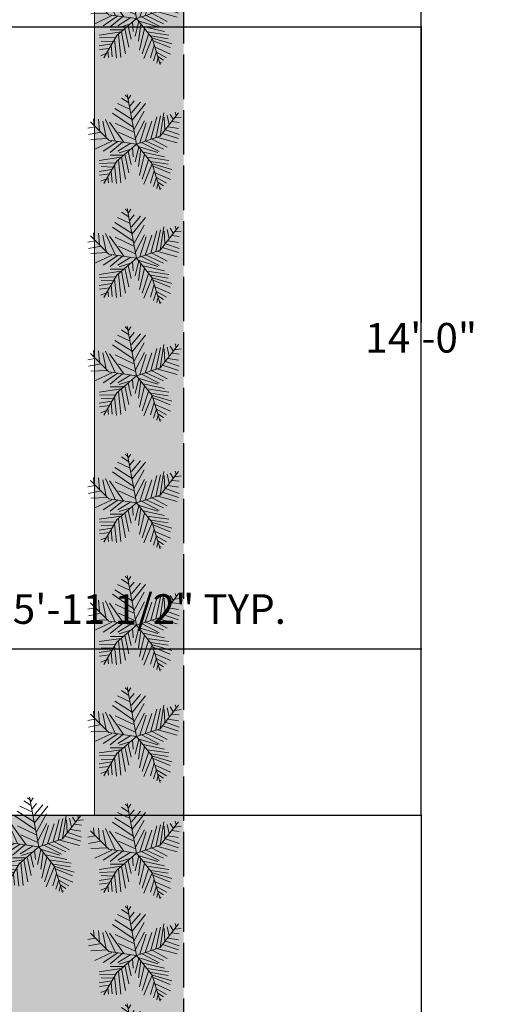
# Model space of a CAD drawing. Units: inches. Extents: x 853 to 1550, y 485 to 1596.
# Tile 8 of 18: x 1418 to 1550, y 768 to 1034. Entities that reach past the tile are written whole.
import ezdxf

# ---------------------------------------------------------------- set-up
doc = ezdxf.new("R2010")
doc.units = ezdxf.units.IN
doc.header["$MEASUREMENT"] = 0
doc.linetypes.add('ACAD_ISO02W100', pattern=[15, 12, -3])
for name, color, linetype, lineweight in [('A-ANNO-DIMS', 2, 'Continuous', 18), ('C-PROP', 8, 'ACAD_ISO02W100', 25), ('L-PLNT-TREE', 106, 'Continuous', 13), ('lawn', 106, 'Continuous', 18)]:
    doc.layers.add(name, color=color, linetype=linetype, lineweight=lineweight)
doc.layers.add('L-PLNT-PATT', color=85, linetype='Continuous', lineweight=13, true_color=0x58ba48)
doc.styles.get("Standard").update_dxf_attribs({"font": 'arial.ttf'})
doc.dimstyles.get("Standard").update_dxf_attribs({"dimtxt": 8, "dimasz": 0.18, "dimexe": 0.18, "dimexo": 0.0625, "dimgap": 0.09, "dimtad": 0, "dimtih": 1, "dimtoh": 1, "dimzin": 0, "dimdsep": 46, "dimlunit": 3, "dimtxsty": 'Standard', "dimcen": 0.09, "dimadec": 0, "dimazin": 0, "dimtfac": 1, "dimtofl": 0, "dimtmove": 0, "dimatfit": 3, "dimfxl": 1, "dimtolj": 1, "dimtzin": 0, "dimarcsym": 0})

# ---------------------------------------------------------------- blocks, each defined once
blk = doc.blocks.new('*U18')
for p, q in [((0, 0), (-10.5, 57)), ((-7.288, 39.707), (-21.778, 46.673)), ((-8.737, 47.138), (-17.069, 52.711)), ((-10.186, 53.64), (-13.084, 55.962)), ((-9.099, 51.782), (-6.563, 55.962)), ((-7.65, 43.423), (-2.578, 49.46)), ((-5.839, 35.992), (4.667, 48.067)), ((-5.114, 27.632), (10.463, 46.673)), ((-3.665, 19.273), (-27.574, 35.527)), ((-5.114, 28.097), (-24.676, 40.636)), ((-2.941, 16.486), (8.652, 37.85)), ((27, 9), (48, 36)), ((27.127, 9.056), (31.112, 35.992)), ((38.719, 34.134), (41.979, 28.561)), ((44.153, 36.456), (45.239, 32.741)), ((-31.5, 4.5), (-52.5, 25.5)), ((-48.585, 21.131), (-49.309, 29.026)), ((-43.513, 28.561), (-42.427, 15.558)), ((-38.442, 26.239), (-34.819, 7.663)), ((-35.544, 28.097), (-24.314, 3.947)), ((-14.533, 2.09), (-30.834, 25.31)), ((-24.314, 23.917), (-2.941, 13.7)), ((-1.129, 6.734), (9.014, 26.704)), ((3.942, 1.625), (11.187, 24.381)), ((10.101, 3.483), (17.708, 26.239)), ((16.259, 5.805), (23.142, 31.348)), ((22.055, 7.198), (27.489, 32.277)), ((31.836, 30.883), (32.561, 16.486)), ((35.096, 32.741), (37.27, 22.524)), ((40.53, 25.775), (48.862, 24.846)), ((43.791, 29.954), (51.036, 30.883)), ((-47.498, 19.737), (-55.83, 18.344)), ((-40.615, 13.7), (-55.105, 10.913)), ((-20.691, 13.7), (-1.129, 4.876)), ((29.662, 12.307), (48.137, 6.269)), ((33.285, 16.486), (48.862, 10.913)), ((36.183, 19.737), (48.137, 17.88)), ((-33.37, 6.269), (-52.207, 5.34)), ((-28.299, 3.483), (-47.86, -5.805)), ((-21.416, 3.018), (-38.079, -8.128)), ((0, 0), (-31.5, 4.5)), ((-15.982, 2.09), (-30.11, -9.521)), ((0, 0), (-22.5, -19.5)), ((-6.563, 1.161), (-21.416, -8.128)), ((0, 0), (27, 9)), ((0, 0), (18, -22.5)), ((6.478, 1.625), (26.04, -8.592)), ((11.187, 3.483), (30.749, -5.805)), ((18.07, 5.805), (35.096, -3.483)), ((24.229, 7.663), (46.688, 1.625)), ((-6.563, -5.805), (-19.967, -9.985)), ((-9.461, -8.592), (-6.201, -23.453)), ((-4.752, -3.483), (-3.665, -14.629)), ((2.493, -3.019), (-1.491, -20.202)), ((1.769, -2.555), (24.229, -9.521)), ((5.029, -6.27), (2.131, -25.775)), ((7.565, -9.056), (32.198, -14.629)), ((-17.431, -15.094), (-42.789, -18.809)), ((-24.314, -21.596), (-42.427, -22.06)), ((-22.5, -19.5), (-37.5, -45)), ((-15.257, -12.772), (-30.11, -12.772)), ((-20.691, -18.345), (-17.793, -44.352)), ((-17.069, -15.094), (-12.721, -40.172)), ((-13.446, -11.378), (-8.737, -32.741)), ((9.014, -11.378), (3.58, -35.992)), ((14.085, -16.951), (6.478, -40.172)), ((18.07, -22.524), (8.289, -45.745)), ((12.274, -15.094), (36.907, -18.809)), ((16.259, -19.738), (36.183, -22.989)), ((18, -22.5), (27, -52.5)), ((18.433, -22.524), (40.53, -29.026)), ((-28.299, -29.026), (-42.789, -31.348)), ((-26.849, -26.24), (-40.253, -25.775)), ((-29.023, -30.884), (-27.936, -43.887)), ((-25.038, -23.918), (-22.865, -45.281)), ((20.244, -30.419), (15.897, -44.816)), ((19.157, -25.311), (38.719, -33.206)), ((21.331, -32.741), (39.081, -40.636)), ((-30.834, -34.135), (-42.427, -35.528)), ((-34.457, -39.708), (-40.978, -42.494)), ((-32.646, -36.921), (-31.921, -44.352)), ((22.78, -37.85), (19.519, -48.532)), ((22.78, -38.314), (34.372, -44.816)), ((24.591, -43.423), (30.749, -47.603)), ((24.591, -45.745), (23.142, -50.854)), ((26.764, -49.925), (28.213, -50.854))]:
    blk.add_line(p, q)
blk = doc.blocks.new('*D41')
at = {"layer": 'A-ANNO-DIMS', "color": 0, "lineweight": -2, "transparency": 16777216}
for p, q in [((1293.81, 863.69), (1293.81, 874.52)), ((1293.99, 874.34), (1365.06, 874.34)), ((1365.24, 863.69), (1365.24, 874.52)), ((1365.24, 874.34), (1365.42, 874.34))]:
    blk.add_line(p, q, dxfattribs=at)
at = {"layer": 'A-ANNO-DIMS', "color": 0, "transparency": 16777216}
for points in [[(1293.99, 874.37), (1293.99, 874.31), (1293.81, 874.34)], [(1365.06, 874.37), (1365.06, 874.31), (1365.24, 874.34)]]:
    blk.add_solid(points, dxfattribs=at)
at = {"layer": 'Defpoints', "color": 0, "transparency": 16777216}
for p in [(1365.24, 874.34), (1293.81, 863.63), (1365.24, 863.63)]:
    blk.add_point(p, dxfattribs=at)
at = {"layer": 'A-ANNO-DIMS', "color": 0, "transparency": 16777216, "insert": (1428.56, 874.34), "char_height": 8, "attachment_point": 5}
blk.add_mtext('\\A1;WINDOW 5\'-11 1/2" TYP.', dxfattribs=at)
blk = doc.blocks.new('*D75')
at = {"layer": 'A-ANNO-DIMS', "color": 0, "lineweight": -2, "transparency": 16777216}
for p, q in [((1405, 1031.63), (1526.24, 1031.63)), ((1526.06, 1031.45), (1526.06, 951.8)), ((1526.06, 863.81), (1526.06, 943.45)), ((1405, 863.63), (1526.24, 863.63))]:
    blk.add_line(p, q, dxfattribs=at)
at = {"layer": 'A-ANNO-DIMS', "color": 0, "transparency": 16777216}
for points in [[(1526.03, 1031.45), (1526.09, 1031.45), (1526.06, 1031.63)], [(1526.03, 863.81), (1526.09, 863.81), (1526.06, 863.63)]]:
    blk.add_solid(points, dxfattribs=at)
at = {"layer": 'Defpoints', "color": 0, "transparency": 16777216}
for p in [(1404.94, 1031.63), (1526.06, 1031.63), (1404.94, 863.63)]:
    blk.add_point(p, dxfattribs=at)
at = {"layer": 'A-ANNO-DIMS', "color": 0, "transparency": 16777216, "insert": (1526.06, 947.63), "char_height": 8, "attachment_point": 5}
blk.add_mtext('\\A1;14\'-0"', dxfattribs=at)
blk = doc.blocks.new('*D79')
at = {"layer": 'A-ANNO-DIMS', "color": 0, "lineweight": -2, "transparency": 16777216}
for p, q in [((1438, 1450.13), (1526.24, 1450.13)), ((1526.06, 1449.95), (1526.06, 1138.61)), ((1526.06, 818.81), (1526.06, 1130.15)), ((1438, 818.63), (1526.24, 818.63))]:
    blk.add_line(p, q, dxfattribs=at)
at = {"layer": 'A-ANNO-DIMS', "color": 0, "transparency": 16777216}
for points in [[(1526.03, 1449.95), (1526.09, 1449.95), (1526.06, 1450.13)], [(1526.03, 818.81), (1526.09, 818.81), (1526.06, 818.63)]]:
    blk.add_solid(points, dxfattribs=at)
at = {"layer": 'Defpoints', "color": 0, "transparency": 16777216}
for p in [(1437.94, 1450.13), (1526.06, 1450.13), (1437.94, 818.63)]:
    blk.add_point(p, dxfattribs=at)
at = {"layer": 'A-ANNO-DIMS', "color": 0, "transparency": 16777216, "insert": (1526.06, 1134.38), "char_height": 8, "attachment_point": 5}
blk.add_mtext('\\A1;52\'-7 1/2"', dxfattribs=at)
blk = doc.blocks.new('*D80')
at = {"layer": 'A-ANNO-DIMS', "color": 0, "lineweight": -2, "transparency": 16777216}
for p, q in [((1307.55, 818.63), (1526.24, 818.63)), ((1526.06, 818.45), (1526.06, 755.21)), ((1526.06, 683.5), (1526.06, 746.75)), ((1307.55, 683.32), (1526.24, 683.32))]:
    blk.add_line(p, q, dxfattribs=at)
at = {"layer": 'A-ANNO-DIMS', "color": 0, "transparency": 16777216}
for points in [[(1526.03, 818.45), (1526.09, 818.45), (1526.06, 818.63)], [(1526.03, 683.5), (1526.09, 683.5), (1526.06, 683.32)]]:
    blk.add_solid(points, dxfattribs=at)
at = {"layer": 'Defpoints', "color": 0, "transparency": 16777216}
for p in [(1307.49, 818.63), (1526.06, 818.63), (1307.49, 683.32)]:
    blk.add_point(p, dxfattribs=at)
at = {"layer": 'A-ANNO-DIMS', "color": 0, "transparency": 16777216, "insert": (1526.06, 750.98), "char_height": 8, "attachment_point": 5}
blk.add_mtext('\\A1;11\'-3 1/2"', dxfattribs=at)

msp = doc.modelspace()

# ---------------------------------------------------------------- hatches: boundary and pattern name
at = {"layer": 'L-PLNT-PATT'}
h = msp.add_hatch(color=256, dxfattribs=at)
h.dxf.hatch_style = 1
h.paths.add_polyline_path([(1461.937, 1474.129), (933.937, 1474.129), (933.937, 730.129), (933.937, 622.891), (941.686, 622.891), (941.686, 604.895), (957.937, 604.895), (957.937, 1450.129), (1437.937, 1450.129), (1437.937, 604.895), (1454.646, 604.895), (1454.646, 622.891), (1461.937, 622.891), (1461.937, 734.988)])
h = msp.add_hatch(color=256, dxfattribs=at)
h.dxf.hatch_style = 1
h.paths.add_polyline_path([(1083.746, 765.455), (957.937, 765.455), (957.937, 604.895), (1121.13, 604.895), (1121.13, 618.052), (1135.564, 618.052), (1135.564, 604.895), (1152.247, 604.895), (1152.247, 610.626), (1152.247, 683.324), (1083.746, 683.324)])
h.paths.add_polyline_path([(1437.937, 818.629), (1307.486, 818.629), (1307.486, 683.324), (1249.908, 683.324), (1249.908, 667.104), (1249.908, 604.895), (1266.059, 604.895), (1266.059, 618.052), (1280.493, 618.052), (1280.493, 604.895), (1437.937, 604.895)])

# ---------------------------------------------------------------- linework, layer by layer
at = {"layer": 'C-PROP'}
msp.add_line((1461.937, 1474.129), (1461.937, 730.129), dxfattribs=at)
at = {"layer": 'lawn'}
for p, q in [((1437.937, 1450.129), (1437.937, 818.629)), ((1437.937, 818.629), (1307.486, 818.629)), ((1383.67, 818.629), (1437.937, 818.629))]:
    msp.add_line(p, q, dxfattribs=at)

# ---------------------------------------------------------------- block references
at = {"layer": 'L-PLNT-TREE', "xscale": 0.2357951711934384, "yscale": 0.2357951711934384, "zscale": 0.2357951711934384}
for p in [(1449.245, 1033.851), (1449.245, 999.946), (1449.245, 969.157), (1449.245, 937.353), (1449.245, 903.032), (1449.245, 869.982), (1449.245, 839.897), (1422.886, 810.116), (1449.245, 808.4), (1449.245, 780.777), (1449.245, 754.254)]:
    msp.add_blockref('*U18', p, dxfattribs=at)

# ---------------------------------------------------------------- dimensions: what is measured, and where the dimension line sits
at = {"layer": 'A-ANNO-DIMS'}
for base, p1, p2, picture, middle in [((1526.064, 1450.129), (1437.937, 818.629), (1437.937, 1450.129), '*D79', (1526.064, 1134.379)), ((1526.064, 1031.629), (1404.937, 863.629), (1404.937, 1031.629), '*D75', (1526.064, 947.629)), ((1526.064, 818.629), (1307.486, 683.324), (1307.486, 818.629), '*D80', (1526.064, 750.977))]:
    dim = msp.add_linear_dim(base=base, p1=p1, p2=p2, angle=90, dimstyle='Standard', override={"dimdec": 1, "dimlfac": 1, "dimrnd": 0, "dimzin": 1, "dimdsep": 46, "dimlunit": 4, "dimfrac": 2}, dxfattribs=at)
    dim.commit()
    dim.dimension.update_dxf_attribs({"geometry": picture, "text_midpoint": middle})
dim = msp.add_linear_dim(base=(1365.241, 874.344), p1=(1293.812, 863.629), p2=(1365.241, 863.629), text='WINDOW <> TYP.', dimstyle='Standard', override={"dimdec": 1, "dimlfac": 1, "dimrnd": 0, "dimzin": 1, "dimdsep": 46, "dimlunit": 4, "dimfrac": 2}, dxfattribs=at)
dim.commit()
dim.dimension.update_dxf_attribs({"geometry": '*D41', "text_midpoint": (1428.556, 874.344)})

doc.saveas('drawing.dxf')
